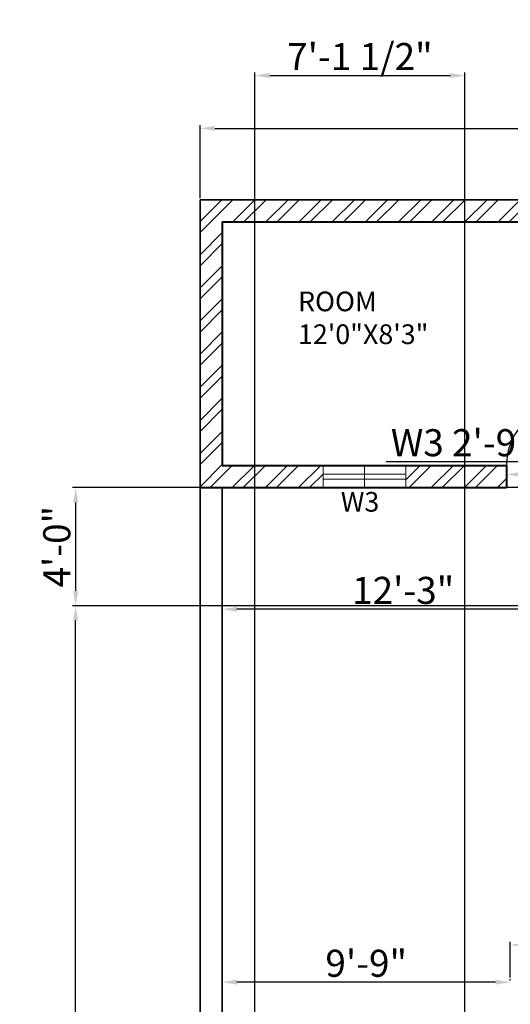
# Model space of a CAD drawing. Units: inches. Extents: x 2069 to 3028, y 691 to 1726.
# Tile 7 of 10: x 2069 to 2268, y 1325 to 1726. Entities that reach past the tile are written whole.
import ezdxf

# ---------------------------------------------------------------- set-up
doc = ezdxf.new("R2010")
doc.units = ezdxf.units.IN
for name, color, linetype, lineweight in [('A-ANNO-DIMS', 2, 'Continuous', 18), ('A-DOOR', 3, 'Continuous', 25), ('A-GLAZ', 4, 'Continuous', 20), ('A-WALL', 7, 'Continuous', 40), ('L-SITE-WALL', 7, 'Continuous', 35)]:
    doc.layers.add(name, color=color, linetype=linetype, lineweight=lineweight)
for name, color, linetype, lineweight, true_color in [('A-ANNO-TEXT', 11, 'Continuous', 18, 0xf27172), ('A-AREA-IDEN', 11, 'Continuous', 25, 0xf27172), ('A-WALL-PATT', 143, 'Continuous', 13, 0x7aafdf)]:
    doc.layers.add(name, color=color, linetype=linetype, lineweight=lineweight, true_color=true_color)
doc.styles.get("Standard").update_dxf_attribs({"font": 'arial.ttf'})
doc.dimstyles.new('ISO-25', dxfattribs={"dimtxt": 11, "dimasz": 6, "dimexe": 1.25, "dimexo": 0.625, "dimtad": 1, "dimlunit": 3, "dimtxsty": 'Standard', "dimcen": 2.5, "dimclrd": 3, "dimclre": 5, "dimclrt": 6, "dimadec": 0, "dimazin": 0, "dimtfac": 1, "dimtmove": 0, "dimatfit": 3, "dimfxl": 1, "dimarcsym": 0})

# ---------------------------------------------------------------- blocks, each defined once
blk = doc.blocks.new('*D20')
at = {"layer": 'A-ANNO-DIMS', "color": 0, "lineweight": -2, "transparency": 16777216}
for p, q in [((2141.95, 1653.01), (2141.95, 1682.68)), ((2147.95, 1681.43), (2840.95, 1681.43)), ((2846.95, 1653.01), (2846.95, 1682.68))]:
    blk.add_line(p, q, dxfattribs=at)
at = {"layer": 'A-ANNO-DIMS', "color": 0, "transparency": 16777216}
for points in [[(2147.95, 1682.43), (2147.95, 1680.43), (2141.95, 1681.43)], [(2840.95, 1682.43), (2840.95, 1680.43), (2846.95, 1681.43)]]:
    blk.add_solid(points, dxfattribs=at)
at = {"layer": 'Defpoints', "color": 0, "transparency": 16777216}
for p in [(2846.95, 1681.43), (2141.95, 1652.39), (2846.95, 1652.39)]:
    blk.add_point(p, dxfattribs=at)
at = {"layer": 'A-ANNO-DIMS', "color": 0, "transparency": 16777216, "insert": (2494.45, 1687.67), "char_height": 11, "attachment_point": 5}
blk.add_mtext('58\'-9"', dxfattribs=at)
blk = doc.blocks.new('*D34')
at = {"layer": 'A-ANNO-DIMS', "color": 0, "lineweight": -2, "transparency": 16777216}
for p, q in [((2150.95, 1335.01), (2150.95, 1335.64)), ((2261.95, 1334.39), (2156.95, 1334.39)), ((2267.95, 1335.01), (2267.95, 1335.64))]:
    blk.add_line(p, q, dxfattribs=at)
at = {"layer": 'A-ANNO-DIMS', "color": 0, "transparency": 16777216}
for points in [[(2156.95, 1335.39), (2156.95, 1333.39), (2150.95, 1334.39)], [(2261.95, 1335.39), (2261.95, 1333.39), (2267.95, 1334.39)]]:
    blk.add_solid(points, dxfattribs=at)
at = {"layer": 'Defpoints', "color": 0, "transparency": 16777216}
for p in [(2150.95, 1334.39), (2150.95, 1334.39), (2267.95, 1334.39)]:
    blk.add_point(p, dxfattribs=at)
at = {"layer": 'A-ANNO-DIMS', "color": 0, "transparency": 16777216, "insert": (2209.45, 1340.63), "char_height": 11, "attachment_point": 5}
blk.add_mtext('9\'-9"', dxfattribs=at)
blk = doc.blocks.new('*D35')
at = {"layer": 'A-ANNO-DIMS', "color": 0, "lineweight": -2, "transparency": 16777216}
for p, q in [((2267.95, 1336.26), (2267.95, 1350.77)), ((2273.95, 1349.52), (2291.95, 1349.52)), ((2297.95, 1336.26), (2297.95, 1350.77)), ((2297.95, 1349.52), (2334.63, 1349.52))]:
    blk.add_line(p, q, dxfattribs=at)
at = {"layer": 'A-ANNO-DIMS', "color": 0, "transparency": 16777216}
for points in [[(2273.95, 1350.52), (2273.95, 1348.52), (2267.95, 1349.52)], [(2291.95, 1350.52), (2291.95, 1348.52), (2297.95, 1349.52)]]:
    blk.add_solid(points, dxfattribs=at)
at = {"layer": 'Defpoints', "color": 0, "transparency": 16777216}
for p in [(2297.95, 1349.52), (2267.95, 1335.64), (2297.95, 1335.64)]:
    blk.add_point(p, dxfattribs=at)
at = {"layer": 'A-ANNO-DIMS', "color": 0, "transparency": 16777216, "insert": (2319.29, 1355.76), "char_height": 11, "attachment_point": 5}
blk.add_mtext('2\'-6"', dxfattribs=at)
blk = doc.blocks.new('*D36')
at = {"layer": 'A-ANNO-DIMS', "color": 0, "lineweight": -2, "transparency": 16777216}
for p, q in [((2150.95, 1486.76), (2150.95, 1484.71)), ((2291.95, 1485.96), (2156.95, 1485.96)), ((2297.95, 1486.76), (2297.95, 1484.71))]:
    blk.add_line(p, q, dxfattribs=at)
at = {"layer": 'A-ANNO-DIMS', "color": 0, "transparency": 16777216}
for points in [[(2156.95, 1486.96), (2156.95, 1484.96), (2150.95, 1485.96)], [(2291.95, 1486.96), (2291.95, 1484.96), (2297.95, 1485.96)]]:
    blk.add_solid(points, dxfattribs=at)
at = {"layer": 'Defpoints', "color": 0, "transparency": 16777216}
for p in [(2150.95, 1487.39), (2150.95, 1485.96), (2297.95, 1487.39)]:
    blk.add_point(p, dxfattribs=at)
at = {"layer": 'A-ANNO-DIMS', "color": 0, "transparency": 16777216, "insert": (2224.45, 1492.21), "char_height": 11, "attachment_point": 5}
blk.add_mtext('12\'-3"', dxfattribs=at)
blk = doc.blocks.new('DOOR-SWING-24IN')
for p, q in [((-1, 0), (-1, 24)), ((0, 0), (0, 24))]:
    blk.add_line(p, q)
blk.add_arc((-0.5, 0.5), 23.51, 88.7811, 181.2189)
blk = doc.blocks.new('WINDOW-SASH-33_6IN')
for p, q in [((0, 0), (33.6, 0)), ((0, -2), (33.6, -2))]:
    blk.add_line(p, q)
blk = doc.blocks.new('*D60')
at = {"layer": 'A-ANNO-DIMS', "color": 3, "lineweight": -2, "transparency": 16777216}
for p, q in [((2345.25, 1545.93), (2217.55, 1545.93)), ((2372.85, 1545.93), (2351.25, 1545.93))]:
    blk.add_line(p, q, dxfattribs=at)
at = {"layer": 'A-ANNO-DIMS', "color": 5, "lineweight": -2, "transparency": 16777216}
for p, q in [((2345.25, 1541.51), (2345.25, 1547.18)), ((2378.85, 1541.51), (2378.85, 1547.18))]:
    blk.add_line(p, q, dxfattribs=at)
at = {"layer": 'A-ANNO-DIMS', "color": 3, "transparency": 16777216}
for points in [[(2351.25, 1546.93), (2351.25, 1544.93), (2345.25, 1545.93)], [(2372.85, 1546.93), (2372.85, 1544.93), (2378.85, 1545.93)]]:
    blk.add_solid(points, dxfattribs=at)
at = {"layer": 'Defpoints', "color": 0, "transparency": 16777216}
for p in [(2345.25, 1545.93), (2345.25, 1540.89), (2378.85, 1540.89)]:
    blk.add_point(p, dxfattribs=at)
at = {"layer": 'A-ANNO-DIMS', "color": 6, "transparency": 16777216, "insert": (2278.4, 1552.24), "char_height": 11, "attachment_point": 5}
blk.add_mtext('W3 2\'-9 1/2" TYP.', dxfattribs=at)
blk = doc.blocks.new('*D62')
at = {"layer": 'A-ANNO-DIMS', "color": 5, "lineweight": -2, "transparency": 16777216}
for p, q in [((2266.31, 1543.76), (2266.31, 1539.52)), ((2290.45, 1543.76), (2290.45, 1539.52))]:
    blk.add_line(p, q, dxfattribs=at)
at = {"layer": 'A-ANNO-DIMS', "color": 3, "lineweight": -2, "transparency": 16777216}
for p, q in [((2272.31, 1540.77), (2284.45, 1540.77)), ((2290.45, 1540.77), (2388.12, 1540.77))]:
    blk.add_line(p, q, dxfattribs=at)
at = {"layer": 'A-ANNO-DIMS', "color": 3, "transparency": 16777216}
for points in [[(2272.31, 1541.77), (2272.31, 1539.77), (2266.31, 1540.77)], [(2284.45, 1541.77), (2284.45, 1539.77), (2290.45, 1540.77)]]:
    blk.add_solid(points, dxfattribs=at)
at = {"layer": 'Defpoints', "color": 0, "transparency": 16777216}
for p in [(2266.31, 1544.39), (2290.45, 1544.39), (2290.45, 1540.77)]:
    blk.add_point(p, dxfattribs=at)
at = {"layer": 'A-ANNO-DIMS', "color": 6, "transparency": 16777216, "insert": (2342.28, 1547.01), "char_height": 11, "attachment_point": 5}
blk.add_mtext('D2 2\'-0" TYP.', dxfattribs=at)
blk = doc.blocks.new('*D87')
at = {"layer": 'A-ANNO-DIMS', "color": 5, "lineweight": -2, "transparency": 16777216}
for p, q in [((2297.33, 1487.39), (2090.2, 1487.39)), ((2297.33, 903.89), (2090.2, 903.89))]:
    blk.add_line(p, q, dxfattribs=at)
at = {"layer": 'A-ANNO-DIMS', "color": 3, "lineweight": -2, "transparency": 16777216}
blk.add_line((2091.45, 909.89), (2091.45, 1481.39), dxfattribs=at)
at = {"layer": 'A-ANNO-DIMS', "color": 3, "transparency": 16777216}
for points in [[(2090.45, 1481.39), (2092.45, 1481.39), (2091.45, 1487.39)], [(2090.45, 909.89), (2092.45, 909.89), (2091.45, 903.89)]]:
    blk.add_solid(points, dxfattribs=at)
at = {"layer": 'Defpoints', "color": 0, "transparency": 16777216}
for p in [(2091.45, 1487.39), (2297.95, 1487.39), (2297.95, 903.89)]:
    blk.add_point(p, dxfattribs=at)
at = {"layer": 'A-ANNO-DIMS', "color": 6, "transparency": 16777216, "insert": (2085.14, 1195.64), "char_height": 11, "attachment_point": 5, "rotation": 90}
blk.add_mtext('48\'-7 1/2"', dxfattribs=at)
blk = doc.blocks.new('*D91')
at = {"layer": 'A-ANNO-DIMS', "color": 5, "lineweight": -2, "transparency": 16777216}
for p, q in [((2289.83, 1535.39), (2090.2, 1535.39)), ((2297.33, 1487.39), (2090.2, 1487.39))]:
    blk.add_line(p, q, dxfattribs=at)
at = {"layer": 'A-ANNO-DIMS', "color": 3, "lineweight": -2, "transparency": 16777216}
blk.add_line((2091.45, 1529.39), (2091.45, 1493.39), dxfattribs=at)
at = {"layer": 'A-ANNO-DIMS', "color": 3, "transparency": 16777216}
for points in [[(2090.45, 1529.39), (2092.45, 1529.39), (2091.45, 1535.39)], [(2090.45, 1493.39), (2092.45, 1493.39), (2091.45, 1487.39)]]:
    blk.add_solid(points, dxfattribs=at)
at = {"layer": 'Defpoints', "color": 0, "transparency": 16777216}
for p in [(2290.45, 1535.39), (2091.45, 1487.39), (2297.95, 1487.39)]:
    blk.add_point(p, dxfattribs=at)
at = {"layer": 'A-ANNO-DIMS', "color": 6, "transparency": 16777216, "insert": (2085.21, 1511.39), "char_height": 11, "attachment_point": 5, "rotation": 90}
blk.add_mtext('4\'-0"', dxfattribs=at)
blk = doc.blocks.new('*D94')
at = {"layer": 'A-ANNO-DIMS', "color": 5, "lineweight": -2, "transparency": 16777216}
for p, q in [((2164.26, 1320.51), (2164.26, 1704.14)), ((2249.51, 1318.68), (2249.51, 1704.14))]:
    blk.add_line(p, q, dxfattribs=at)
at = {"layer": 'A-ANNO-DIMS', "color": 3, "lineweight": -2, "transparency": 16777216}
blk.add_line((2170.26, 1702.89), (2243.51, 1702.89), dxfattribs=at)
at = {"layer": 'A-ANNO-DIMS', "color": 3, "transparency": 16777216}
for points in [[(2170.26, 1703.89), (2170.26, 1701.89), (2164.26, 1702.89)], [(2243.51, 1703.89), (2243.51, 1701.89), (2249.51, 1702.89)]]:
    blk.add_solid(points, dxfattribs=at)
at = {"layer": 'Defpoints', "color": 0, "transparency": 16777216}
for p in [(2249.51, 1702.89), (2164.26, 1319.89), (2249.51, 1318.06)]:
    blk.add_point(p, dxfattribs=at)
at = {"layer": 'A-ANNO-DIMS', "color": 6, "transparency": 16777216, "insert": (2206.88, 1709.2), "char_height": 11, "attachment_point": 5}
blk.add_mtext('7\'-1 1/2"', dxfattribs=at)

msp = doc.modelspace()

# ---------------------------------------------------------------- hatches: boundary and pattern name
at = {"layer": 'A-WALL-PATT'}
h = msp.add_hatch(dxfattribs=at)
h.set_pattern_fill('ANSI32', color=256)
h.paths.add_polyline_path([(2609.951, 1652.387), (2141.951, 1652.387), (2141.951, 1535.387), (2191.901, 1535.387), (2191.901, 1544.387), (2150.951, 1544.387), (2150.951, 1643.387), (2294.951, 1643.387), (2294.951, 1544.387), (2290.451, 1544.387), (2290.451, 1535.387), (2345.247, 1535.387), (2345.247, 1544.387), (2303.951, 1544.387), (2303.951, 1643.387), (2447.951, 1643.387), (2447.951, 1544.387), (2444.144, 1544.387), (2444.144, 1535.387), (2461.327, 1535.387), (2461.327, 1544.387), (2456.951, 1544.387), (2456.951, 1643.387), (2600.951, 1643.387), (2600.951, 1544.387), (2559.939, 1544.387), (2559.939, 1535.387), (2609.951, 1535.387)])
h.paths.add_polyline_path([(2266.451, 1544.387), (2225.501, 1544.387), (2225.501, 1535.387), (2266.451, 1535.387)], flags=17)
h.paths.add_polyline_path([(2420.144, 1544.387), (2378.847, 1544.387), (2378.847, 1535.387), (2420.144, 1535.387)], flags=17)
h.paths.add_polyline_path([(2526.339, 1544.387), (2485.327, 1544.387), (2485.327, 1535.387), (2526.339, 1535.387)], flags=17)

# ---------------------------------------------------------------- linework, layer by layer
at = {"layer": 'A-GLAZ'}
for p, q in [((2191.901, 1544.387), (2191.901, 1535.387)), ((2208.701, 1544.387), (2208.701, 1535.387)), ((2225.501, 1544.387), (2225.501, 1535.387))]:
    msp.add_line(p, q, dxfattribs=at)
at = {"layer": 'A-WALL'}
for p, q in [((2150.951, 1643.387), (2294.951, 1643.387)), ((2150.951, 1643.387), (2150.951, 1544.387)), ((2150.951, 1544.387), (2266.451, 1544.387)), ((2266.451, 1544.387), (2266.451, 1535.387)), ((2141.951, 1535.387), (2266.451, 1535.387))]:
    msp.add_line(p, q, dxfattribs=at)
at = {"layer": 'L-SITE-WALL'}
for p, q in [((2141.951, 1652.387), (2846.951, 1652.387)), ((2141.951, 1652.387), (2141.951, 737.387)), ((2150.951, 1535.387), (2150.951, 746.387))]:
    msp.add_line(p, q, dxfattribs=at)

# ---------------------------------------------------------------- block references
at = {"layer": 'A-DOOR'}
msp.add_blockref('DOOR-SWING-24IN', (2290.451, 1544.387), dxfattribs=at)
at = {"layer": 'A-GLAZ'}
msp.add_blockref('WINDOW-SASH-33_6IN', (2191.901, 1540.887), dxfattribs=at)

# ---------------------------------------------------------------- texts
at = {"layer": 'A-ANNO-TEXT', "insert": (2199.115, 1533.634), "char_height": 8, "attachment_point": 1}
msp.add_mtext_dynamic_manual_height_columns('{\\fArial|b1|i0|c0|p34;W3}', width=34.05605, gutter_width=12.5, heights=[0], dxfattribs=at)
at = {"layer": 'A-AREA-IDEN', "insert": (2181.743, 1615.089), "char_height": 8, "attachment_point": 1}
msp.add_mtext_dynamic_manual_height_columns('ROOM\\P12\'0"X8\'3"', width=119.20948, gutter_width=12.5, heights=[0], dxfattribs=at)

# ---------------------------------------------------------------- dimensions: what is measured, and where the dimension line sits
at = {"layer": 'A-ANNO-DIMS'}
for base, p1, p2, override, picture, middle in [((2249.51, 1702.887), (2164.257, 1319.887), (2249.51, 1318.058), {"dimdec": 1, "dimlfac": 1, "dimrnd": 0, "dimzin": 1, "dimdsep": 46, "dimlunit": 4, "dimfrac": 2}, '*D94', (2206.884, 1709.199)), ((2846.951, 1681.427), (2141.951, 1652.387), (2846.951, 1652.387), {"dimclrd": 0, "dimclre": 0, "dimclrt": 0}, '*D20', (2494.451, 1687.669)), ((2150.951, 1485.965), (2297.951, 1487.387), (2150.951, 1487.387), {"dimclrd": 0, "dimclre": 0, "dimclrt": 0}, '*D36', (2224.451, 1492.21)), ((2297.951, 1349.515), (2267.951, 1335.637), (2297.951, 1335.637), {"dimclrd": 0, "dimclre": 0, "dimclrt": 0}, '*D35', (2319.29, 1355.757)), ((2150.951, 1334.387), (2267.951, 1334.387), (2150.951, 1334.387), {"dimclrd": 0, "dimclre": 0, "dimclrt": 0}, '*D34', (2209.451, 1340.628))]:
    dim = msp.add_linear_dim(base=base, p1=p1, p2=p2, dimstyle='ISO-25', override=override, dxfattribs=at)
    dim.commit()
    dim.dimension.update_dxf_attribs({"geometry": picture, "text_midpoint": middle})
dim = msp.add_linear_dim(base=(2345.247, 1545.927), p1=(2378.847, 1540.887), p2=(2345.247, 1540.887), angle=180, text='W3 <> TYP.', dimstyle='ISO-25', override={"dimdec": 1, "dimlfac": 1, "dimrnd": 0, "dimzin": 1, "dimdsep": 46, "dimlunit": 4, "dimfrac": 2}, dxfattribs=at)
dim.commit()
dim.dimension.update_dxf_attribs({"geometry": '*D60', "text_midpoint": (2278.396, 1552.243)})
dim = msp.add_linear_dim(base=(2290.451, 1540.766), p1=(2266.315, 1544.387), p2=(2290.451, 1544.387), text='D2 <> TYP.', dimstyle='ISO-25', override={"dimdec": 1, "dimlfac": 1, "dimrnd": 0, "dimzin": 1, "dimdsep": 46, "dimlunit": 4, "dimfrac": 2}, dxfattribs=at)
dim.commit()
dim.dimension.update_dxf_attribs({"geometry": '*D62', "text_midpoint": (2342.284, 1547.007)})
for p1, picture, middle in [((2290.451, 1535.387), '*D91', (2085.21, 1511.387)), ((2297.951, 903.887), '*D87', (2085.139, 1195.637))]:
    dim = msp.add_linear_dim(base=(2091.451, 1487.387), p1=p1, p2=(2297.951, 1487.387), angle=90, dimstyle='ISO-25', override={"dimdec": 1, "dimlfac": 1, "dimrnd": 0, "dimzin": 1, "dimdsep": 46, "dimlunit": 4, "dimfrac": 2}, dxfattribs=at)
    dim.commit()
    dim.dimension.update_dxf_attribs({"geometry": picture, "text_midpoint": middle})

doc.saveas('drawing.dxf')
